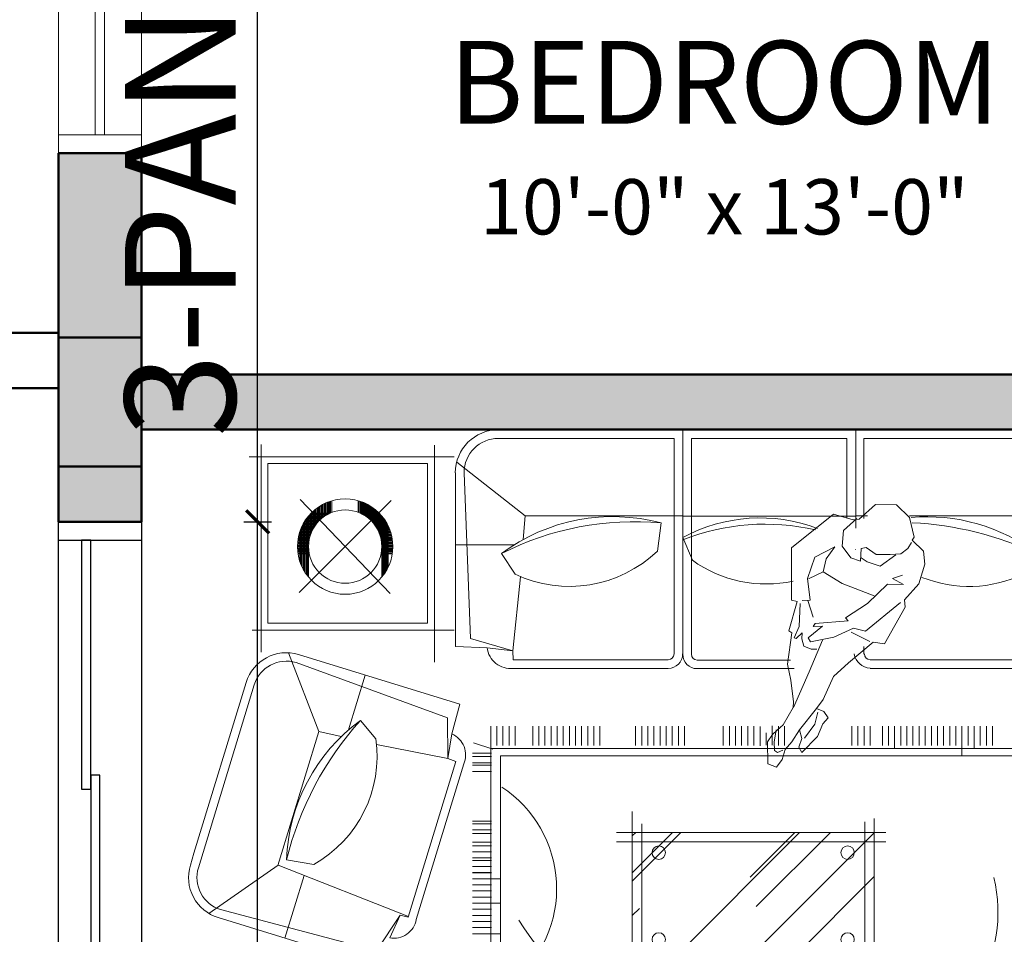
# Model space of a CAD drawing. Units: inches. Extents: x 375 to 1122, y 27 to 1069.
# Tile 69 of 155: x 494 to 601, y 400 to 499. Entities that reach past the tile are written whole.
import ezdxf

# ---------------------------------------------------------------- set-up
doc = ezdxf.new("R2010")
doc.units = ezdxf.units.IN
for name, color, linetype, lineweight in [('A-ANNO-DIMS', 2, 'Continuous', 18), ('A-AREA-IDEN', 7, 'Continuous', 18), ('A-COLS-PATT', 10, 'Continuous', 13), ('A-WALL-PATT', 252, 'Continuous', 13), ('Columns', 10, 'Continuous', 50), ('Doors', 150, 'Continuous', 25), ('Furniture', 30, 'Continuous', 18), ('Walls', 250, 'Continuous', 50), ('Windows', 122, 'Continuous', 18)]:
    doc.layers.add(name, color=color, linetype=linetype, lineweight=lineweight)
doc.styles.get("Standard").update_dxf_attribs({"font": 'arial.ttf'})
doc.dimstyles.new('ISO-25', dxfattribs={"dimtxt": 12, "dimasz": 2.5, "dimexe": 1.5, "dimexo": 1.5, "dimtad": 1, "dimdec": 1, "dimlunit": 3, "dimtxsty": 'Standard', "dimblk": 'ARCHTICK', "dimcen": 2.5, "dimadec": 0, "dimazin": 0, "dimtfac": 1, "dimtdec": 1, "dimtmove": 0, "dimatfit": 3, "dimfxl": 1.5, "dimfxlon": 1, "dimarcsym": 0})

# ---------------------------------------------------------------- blocks, each defined once
blk = doc.blocks.new('A$C4DC51D13')
for p, q in [((3265.3, 2996.2), (1188.4, 2996.2)), ((1895.2, 2134), (1895.2, 2996.2)), ((2559.6, 2996.2), (2559.6, 2617.8)), ((1188.4, 2962.7), (1862.1, 2962.7)), ((1862.1, 2134), (1862.1, 2962.7)), ((1928.3, 2961.6), (2524.2, 2961.6)), ((1928.3, 2134), (1928.3, 2961.6)), ((2524.2, 2961.6), (2524.2, 2658.6)), ((2590.4, 2962.7), (2590.4, 2654.5)), ((3265.3, 2962.7), (2590.4, 2962.7)), ((277.4, 2939.6), (277.4, 2141.8)), ((943, 2103.5), (943, 2936.7)), ((1018.2, 2892.3), (232.2, 2892.3)), ((1290.4, 2664.8), (1028, 2870.9)), ((304, 2865.7), (304, 2253.3)), ((916.4, 2865.7), (304, 2865.7)), ((916.4, 2253.3), (916.4, 2865.7)), ((1022.9, 2163.8), (1022.9, 2830.3)), ((1056, 2830.3), (1081, 2194.8)), ((423.7, 2370.8), (776.6, 2723.7)), ((427.4, 2727.4), (772.8, 2367.1)), ((540.2, 2674.6), (540.2, 2720.2)), ((544.4, 2676.5), (544.4, 2721.6)), ((548.7, 2678.2), (548.7, 2722.9)), ((650.1, 2678.8), (650.1, 2723.3)), ((654.3, 2677.1), (654.3, 2722)), ((658.6, 2675.2), (658.6, 2720.7)), ((476.8, 2615), (476.8, 2682.5)), ((481, 2622.2), (481, 2686.2)), ((485.3, 2628.5), (485.3, 2689.7)), ((489.5, 2634.2), (489.5, 2693)), ((493.7, 2639.3), (493.7, 2696.1)), ((497.9, 2644), (497.9, 2699.1)), ((502.2, 2648.3), (502.2, 2701.8)), ((506.4, 2652.2), (506.4, 2704.4)), ((510.6, 2655.8), (510.6, 2706.9)), ((514.9, 2659.2), (514.9, 2709.2)), ((519.1, 2662.3), (519.1, 2711.3)), ((523.3, 2665.1), (523.3, 2713.4)), ((527.5, 2667.8), (527.5, 2715.2)), ((531.8, 2670.2), (531.8, 2717)), ((536, 2672.5), (536, 2718.7)), ((662.8, 2673.2), (662.8, 2719.2)), ((667, 2671), (667, 2717.6)), ((668.5, 2670.2), (668.5, 2717)), ((671.2, 2668.6), (671.2, 2715.9)), ((672.7, 2667.8), (672.7, 2715.2)), ((675.5, 2666.1), (675.5, 2714)), ((676.9, 2665.1), (676.9, 2713.4)), ((679.7, 2663.3), (679.7, 2712)), ((681.1, 2662.3), (681.1, 2711.3)), ((683.9, 2660.3), (683.9, 2709.9)), ((685.4, 2659.2), (685.4, 2709.2)), ((688.1, 2657), (688.1, 2707.7)), ((689.6, 2655.8), (689.6, 2706.9)), ((692.4, 2653.5), (692.4, 2705.3)), ((693.8, 2652.2), (693.8, 2704.4)), ((696.6, 2649.6), (696.6, 2702.7)), ((698, 2648.3), (698, 2701.8)), ((700.8, 2645.5), (700.8, 2700)), ((702.3, 2644), (702.3, 2699.1)), ((705, 2641), (705, 2697.2)), ((706.5, 2639.3), (706.5, 2696.1)), ((709.3, 2636), (709.3, 2694.1)), ((710.7, 2634.2), (710.7, 2693)), ((713.5, 2630.5), (713.5, 2690.9)), ((714.9, 2628.5), (714.9, 2689.7)), ((717.7, 2624.4), (717.7, 2687.4)), ((719.2, 2622.2), (719.2, 2686.2)), ((722, 2617.6), (722, 2683.8)), ((723.4, 2615), (723.4, 2682.5)), ((446.1, 2646.1), (500, 2646.1)), ((447.2, 2446.7), (447.2, 2647.8)), ((448.9, 2650.4), (504.4, 2650.4)), ((451.5, 2440.6), (451.5, 2654)), ((451.9, 2654.6), (509.2, 2654.6)), ((455.1, 2658.8), (514.4, 2658.8)), ((455.7, 2434.9), (455.7, 2659.6)), ((458.4, 2663.1), (520.2, 2663.1)), ((459.9, 2558.8), (459.9, 2664.9)), ((462, 2667.3), (526.7, 2667.3)), ((464.1, 2583.3), (464.1, 2669.7)), ((465.8, 2671.5), (534.1, 2671.5)), ((468.4, 2596.6), (468.4, 2674.3)), ((469.8, 2675.7), (542.8, 2675.7)), ((472.6, 2606.7), (472.6, 2678.5)), ((489.5, 2667.3), (489.5, 2633.5)), ((657.4, 2675.7), (730.4, 2675.7)), ((734.5, 2671.5), (666.1, 2671.5)), ((666.1, 2671.5), (734.5, 2671.5)), ((738.2, 2667.3), (673.5, 2667.3)), ((673.5, 2667.3), (738.2, 2667.3)), ((741.8, 2663.1), (680, 2663.1)), ((680, 2663.1), (741.8, 2663.1)), ((745.2, 2658.8), (685.8, 2658.8)), ((685.8, 2658.8), (745.2, 2658.8)), ((748.3, 2654.6), (691, 2654.6)), ((691, 2654.6), (748.3, 2654.6)), ((751.3, 2650.4), (695.8, 2650.4)), ((695.8, 2650.4), (751.3, 2650.4)), ((754.1, 2646.1), (700.2, 2646.1)), ((700.2, 2646.1), (754.1, 2646.1)), ((726.2, 2609.7), (726.2, 2679.9)), ((727.6, 2606.7), (727.6, 2678.5)), ((730.4, 2600.3), (730.4, 2675.7)), ((731.9, 2596.6), (731.9, 2674.3)), ((734.6, 2588.4), (734.6, 2671.3)), ((736.1, 2583.3), (736.1, 2669.7)), ((738.9, 2570.4), (738.9, 2666.6)), ((740.3, 2558.8), (740.3, 2664.9)), ((743.1, 2433.1), (743.1, 2661.5)), ((744.5, 2434.9), (744.5, 2659.6)), ((747.3, 2438.6), (747.3, 2656)), ((748.8, 2440.6), (748.8, 2654)), ((751.5, 2444.5), (751.5, 2650)), ((753, 2446.7), (753, 2647.8)), ((1283.3, 2574.2), (1290.4, 2664.8)), ((1290.4, 2664.8), (1894.7, 2664.8)), ((1895.2, 2663.7), (2557.3, 2663.7)), ((2603.6, 2664.8), (2559, 2664.8)), ((3163.3, 2664.8), (2764.7, 2664.8)), ((427.5, 2608.1), (473.3, 2608.1)), ((429.1, 2612.3), (475.4, 2612.3)), ((430.3, 2479), (430.3, 2615.5)), ((430.7, 2616.6), (477.7, 2616.6)), ((432.5, 2620.8), (480.2, 2620.8)), ((434.5, 2469.3), (434.5, 2625.2)), ((434.5, 2625), (482.9, 2625)), ((436.5, 2629.2), (485.8, 2629.2)), ((438.7, 2633.5), (488.9, 2633.5)), ((438.8, 2460.9), (438.8, 2633.6)), ((441, 2637.7), (492.3, 2637.7)), ((443, 2453.4), (443, 2641.1)), ((443.5, 2641.9), (496, 2641.9)), ((756.7, 2641.9), (704.2, 2641.9)), ((704.2, 2641.9), (756.7, 2641.9)), ((759.2, 2637.7), (707.9, 2637.7)), ((707.9, 2637.7), (759.2, 2637.7)), ((761.5, 2633.5), (711.3, 2633.5)), ((711.3, 2633.5), (761.5, 2633.5)), ((763.7, 2629.2), (714.4, 2629.2)), ((714.4, 2629.2), (763.7, 2629.2)), ((765.8, 2625), (717.3, 2625)), ((767.7, 2620.8), (720, 2620.8)), ((769.5, 2616.6), (722.5, 2616.6)), ((771.1, 2612.3), (724.8, 2612.3)), ((772.7, 2608.1), (726.9, 2608.1)), ((755.8, 2451.1), (755.8, 2643.5)), ((757.2, 2453.4), (757.2, 2641.1)), ((760, 2458.3), (760, 2636.3)), ((761.4, 2460.9), (761.4, 2633.6)), ((764.2, 2466.3), (764.2, 2628.2)), ((765.7, 2469.3), (765.7, 2625.2)), ((1798, 2530.2), (1812.1, 2637.9)), ((418.5, 2570.1), (461.3, 2570.1)), ((419.1, 2574.3), (462.1, 2574.3)), ((419.8, 2578.5), (462.9, 2578.5)), ((420.6, 2582.7), (464, 2582.7)), ((421.5, 2587), (465.2, 2587)), ((422.5, 2591.2), (466.5, 2591.2)), ((423.6, 2595.4), (467.9, 2595.4)), ((424.8, 2599.7), (469.6, 2599.7)), ((426.1, 2603.9), (471.3, 2603.9)), ((426.1, 2490.7), (426.1, 2603.9)), ((774.1, 2603.9), (728.9, 2603.9)), ((775.4, 2599.7), (730.7, 2599.7)), ((776.6, 2595.4), (732.3, 2595.4)), ((777.7, 2591.2), (733.7, 2591.2)), ((778.7, 2587), (735.1, 2587)), ((779.6, 2582.7), (736.2, 2582.7)), ((780.4, 2578.5), (737.3, 2578.5)), ((781.1, 2574.3), (738.2, 2574.3)), ((781.7, 2570.1), (738.9, 2570.1)), ((1895.5, 2582.2), (1932.3, 2494.6)), ((417.1, 2548.9), (459.4, 2548.9)), ((417.1, 2544.7), (459.5, 2544.7)), ((417.2, 2553.2), (459.6, 2553.2)), ((417.2, 2540.5), (459.6, 2540.5)), ((417.4, 2557.4), (459.8, 2557.4)), ((417.5, 2536.3), (459.9, 2536.3)), ((417.7, 2561.6), (460.2, 2561.6)), ((417.8, 2532), (460.3, 2532)), ((418.1, 2565.8), (460.7, 2565.8)), ((459.9, 2429.7), (459.9, 2535.7)), ((782.2, 2565.8), (739.6, 2565.8)), ((782.5, 2532), (740, 2532)), ((782.5, 2561.6), (740.1, 2561.6)), ((740.3, 2429.7), (740.3, 2535.7)), ((782.8, 2557.4), (740.4, 2557.4)), ((782.8, 2536.3), (740.4, 2536.3)), ((783, 2540.5), (740.6, 2540.5)), ((783, 2553.2), (740.7, 2553.2)), ((783.1, 2548.9), (740.8, 2548.9)), ((783.1, 2544.7), (740.8, 2544.7)), ((1022.9, 2554.4), (1249.6, 2554.4)), ((2559, 2535.8), (2557.3, 2535.8)), ((418.2, 2527.8), (460.8, 2527.8)), ((418.7, 2523.6), (461.4, 2523.6)), ((419.3, 2519.4), (462.2, 2519.4)), ((781, 2519.4), (738, 2519.4)), ((781.6, 2523.6), (738.8, 2523.6)), ((782.1, 2527.8), (739.4, 2527.8)), ((1200, 2520.5), (1251.9, 2440.8)), ((1243.2, 2146.7), (1272.2, 2431.8)), ((304, 2253.3), (916.4, 2253.3)), ((242.9, 2226.7), (1018.2, 2226.7)), ((1081, 2194.8), (1243.2, 2146.7)), ((1145.1, 2159.3), (1022.9, 2163.8)), ((1145.1, 2159.3), (1243.2, 2146.7)), ((2590.4, 2164.3), (2590.4, 2134)), ((498.8, 1837.1), (382.1, 2139.5)), ((1040.3, 1942.9), (421.2, 2132.6)), ((1244.8, 2113), (1243.2, 2146.7)), ((411.8, 2101.9), (992.6, 1890.2)), ((1839.5, 2113), (1244.8, 2113)), ((1839.5, 2079.9), (1244.8, 2079.9)), ((2308.5, 2111.9), (1950.4, 2111.9)), ((2322.1, 2078.8), (1950.4, 2078.8)), ((2614.2, 2113), (3208.9, 2113)), ((2614.2, 2079.9), (3208.9, 2079.9)), ((677.4, 2054.1), (612.9, 1843.6)), ((220.3, 2026), (19.3, 1370.1)), ((251.1, 2016.6), (37.1, 1314.7)), ((1009.7, 1828.1), (1040.3, 1942.9)), ((992.6, 1890.2), (993.4, 1733.4)), ((658.5, 1880), (717.8, 1809.1)), ((1158.3, 1784.3), (1158.3, 1858.2)), ((1181.8, 1784.3), (1181.8, 1858.2)), ((1205.3, 1784.3), (1205.3, 1858.2)), ((1228.8, 1784.3), (1228.8, 1858.2)), ((1252.2, 1784.3), (1252.2, 1858.2)), ((1319.4, 1784.3), (1319.4, 1858.2)), ((1342.9, 1784.3), (1342.9, 1858.2)), ((1366.3, 1784.3), (1366.3, 1858.2)), ((1389.8, 1784.3), (1389.8, 1858.2)), ((1413.3, 1784.3), (1413.3, 1858.2)), ((1436.8, 1784.3), (1436.8, 1858.2)), ((1460.2, 1784.3), (1460.2, 1858.2)), ((1483.7, 1784.3), (1483.7, 1858.2)), ((1507.2, 1784.3), (1507.2, 1858.2)), ((1530.7, 1784.3), (1530.7, 1858.2)), ((1554.1, 1784.3), (1554.1, 1858.2)), ((1577.6, 1784.3), (1577.6, 1858.2)), ((1714.2, 1784.3), (1714.2, 1858.2)), ((1737.6, 1784.3), (1737.6, 1858.2)), ((1761.1, 1784.3), (1761.1, 1858.2)), ((1784.6, 1784.3), (1784.6, 1858.2)), ((1808.1, 1784.3), (1808.1, 1858.2)), ((1831.5, 1784.3), (1831.5, 1858.2)), ((1855, 1784.3), (1855, 1858.2)), ((1878.5, 1784.3), (1878.5, 1858.2)), ((1902, 1784.3), (1902, 1858.2)), ((2050.7, 1784.3), (2050.7, 1858.2)), ((2074.2, 1784.3), (2074.2, 1858.2)), ((2097.7, 1784.3), (2097.7, 1858.2)), ((2121.1, 1784.3), (2121.1, 1858.2)), ((2144.6, 1784.3), (2144.6, 1858.2)), ((2168.1, 1784.3), (2168.1, 1858.2)), ((2191.6, 1782.4), (2191.6, 1856.3)), ((2238.5, 1785.1), (2238.5, 1859)), ((2262, 1784.3), (2262, 1858.2)), ((2285.4, 1784.3), (2285.4, 1858.2)), ((2543.7, 1784.3), (2543.7, 1858.2)), ((2567.1, 1784.3), (2567.1, 1858.2)), ((2590.6, 1784.3), (2590.6, 1858.2)), ((2614.1, 1784.3), (2614.1, 1858.2)), ((2661, 1784.3), (2661, 1858.2)), ((2684.5, 1784.3), (2684.5, 1858.2)), ((2708, 1772.3), (2708, 1858.2)), ((2731.5, 1784.3), (2731.5, 1858.2)), ((2754.9, 1784.3), (2754.9, 1858.2)), ((2778.4, 1784.3), (2778.4, 1858.2)), ((2801.9, 1784.3), (2801.9, 1858.2)), ((2825.4, 1784.3), (2825.4, 1858.2)), ((2848.8, 1784.3), (2848.8, 1858.2)), ((2872.3, 1784.3), (2872.3, 1858.2)), ((2895.8, 1784.3), (2895.8, 1858.2)), ((2919.3, 1784.3), (2919.3, 1858.2)), ((2942.7, 1784.3), (2942.7, 1858.2)), ((2966.2, 1744.8), (2966.2, 1858.2)), ((2989.7, 1784.3), (2989.7, 1858.2)), ((3013.2, 1772.3), (3013.2, 1858.2)), ((3036.6, 1784.3), (3036.6, 1858.2)), ((3060.1, 1784.3), (3060.1, 1858.2)), ((3083.6, 1784.3), (3083.6, 1858.2)), ((498.8, 1837.1), (341.4, 1323.6)), ((584.9, 1817.9), (498.8, 1837.1)), ((1009.7, 1828.1), (993.4, 1733.4)), ((1158.3, 1821.3), (1158.5, 487.7)), ((2215, 1785.7), (2215, 1832.3)), ((993.4, 1733.4), (720.4, 1787.6)), ((1166.1, 1769.7), (1091.8, 1794.5)), ((1162.1, 1754.9), (1088.2, 1754.9)), ((1162.1, 1741.1), (1088.2, 1741.1)), ((3248.4, 1772.3), (1158.5, 1772.3)), ((1196, 511), (1196, 1744.8)), ((1196, 1744.8), (3215.6, 1744.8)), ((1024.2, 1722.3), (842.3, 1125.2)), ((873.1, 1115.8), (1055, 1712.9)), ((1024.2, 1722.3), (993.4, 1733.4)), ((1162.1, 1717.6), (1088.2, 1717.6)), ((1162.1, 1708), (1088.2, 1708)), ((1162.1, 1684.5), (1088.2, 1684.5)), ((1701.7, 1530), (1701.7, 911.2)), ((1162.1, 1492.9), (1088.2, 1492.9)), ((1162.1, 1483.3), (1088.2, 1483.3)), ((1737.7, 1483.1), (1737.7, 911.2)), ((2593.1, 907.9), (2593.1, 1490.3)), ((2629.1, 907.9), (2629.1, 1503.1)), ((1162.1, 1459.8), (1088.2, 1459.8)), ((1162.1, 1446), (1088.2, 1446)), ((2674.6, 1449.9), (1641, 1449.9)), ((1888.1, 1449.9), (1701.7, 1263.5)), ((1856.2, 1449.9), (1701.7, 1295.4)), ((1715.1, 1449.9), (1701.7, 1436.5)), ((2343.3, 1449.9), (1855.3, 961.9)), ((2629.1, 1449), (2142, 961.9)), ((2325.1, 1449.9), (2154.2, 1279.1)), ((2461.6, 1449.9), (2177, 1165.3)), ((1162.1, 1412.8), (1088.2, 1412.8)), ((1162.1, 1399), (1088.2, 1399)), ((2674.6, 1413.9), (1641, 1413.9)), ((6.3, 1324.2), (19.3, 1370.2)), ((1162.1, 1375.5), (1088.2, 1375.5)), ((342.8, 1324.6), (76.7, 1139.6)), ((843, 1127.6), (342.8, 1324.6)), ((479.3, 1327.3), (375.2, 1344.9)), ((1162.1, 1352.1), (1088.2, 1352.1)), ((1162.1, 1342.9), (1088.2, 1342.9)), ((1162.1, 1342.4), (1088.2, 1342.4)), ((369.2, 1044.8), (442.9, 1285.2)), ((1162.1, 1319.4), (1088.2, 1319.4)), ((1162.1, 1318.9), (1088.2, 1318.9)), ((1162.1, 1296), (1088.2, 1296)), ((1162.1, 1295.5), (1088.2, 1295.5)), ((1196, 1272.5), (1088.2, 1272.5)), ((1162.1, 1272), (1088.2, 1272)), ((1162.1, 1249), (1088.2, 1249)), ((1162.1, 1248.5), (1088.2, 1248.5)), ((2629.1, 1280.5), (2310.5, 961.9)), ((1162.1, 1225.5), (1088.2, 1225.5)), ((1162.1, 1202.1), (1088.2, 1202.1)), ((1196, 1178.6), (1088.2, 1178.6)), ((122.4, 1154.1), (719.7, 996.3)), ((719.7, 996.3), (810.6, 1133.2)), ((771, 1045.7), (810.6, 1133.2)), ((842.3, 1125.2), (810.6, 1133.2)), ((1162.1, 1155.1), (1088.2, 1155.1)), ((1728.6, 1158.4), (1701.7, 1131.5)), ((732, 933.5), (112.9, 1123.3)), ((1162.1, 1131.6), (1088.2, 1131.6)), ((1162.1, 1108.2), (1088.2, 1108.2)), ((1162.1, 1084.7), (1088.2, 1084.7)), ((1196, 1061.2), (1088.2, 1061.2))]:
    blk.add_line(p, q)
at = {"linetype": 'ByBlock'}
blk.add_lwpolyline([(2342.9, 1843.9), (2352.5, 1810.4), (2340.1, 1777.7), (2351.8, 1757), (2412.3, 1818), (2433.1, 1866.4), (2453.1, 1889.5), (2436, 1914.7), (2407.6, 1926.2), (2433.7, 1959.9), (2473.1, 2048.3), (2530.6, 2101.1), (2625.9, 2180.3), (2669, 2174.2), (2748.1, 2315.4), (2745.8, 2342.6), (2801.2, 2404.9), (2823.9, 2479.6), (2818.4, 2529.9), (2775.1, 2571.7), (2782.4, 2583.3), (2765.2, 2658.8), (2714.5, 2706.9), (2634.6, 2708.6), (2571.9, 2652.6), (2548.8, 2649.4), (2474, 2672.1), (2312.9, 2542.1), (2312.9, 2341.6), (2333.9, 2336.4), (2302, 2223.9), (2313.6, 2216.6), (2297.4, 2095.7), (2309.3, 2034.9), (2320.2, 1952), (2319.3, 1929.9), (2280.8, 1863.6), (2257.7, 1842.4), (2239.2, 1825.7), (2220.1, 1798.2), (2221.6, 1713.1), (2254.3, 1700.7), (2275.9, 1729.8), (2288.6, 1768), (2313.7, 1797.6)], close=True, dxfattribs=at)
for points in [[(2563.4, 2654.7), (2512.2, 2609.3), (2506.2, 2548.3), (2540.1, 2504.4), (2576.9, 2490.9), (2579.8, 2539.3), (2598.7, 2543.6), (2636.7, 2516.4), (2690.3, 2516.7), (2731.2, 2520.1), (2758.5, 2540.1), (2773, 2563.3)], [(2629.1, 2357.8), (2507, 2405.5), (2433.2, 2450.3), (2445.5, 2500.8), (2478.9, 2546.1), (2402.4, 2506.9), (2373.4, 2424.8), (2384.4, 2341.9), (2352.8, 2340.7)], [(2712.3, 2515.8), (2652.7, 2472.4), (2603.2, 2489), (2580, 2503.6)], [(2738, 2438.2), (2699.2, 2425.4), (2742.4, 2401.4), (2680.4, 2403.2), (2604.1, 2328.3), (2519.2, 2273.3), (2529.8, 2261.8), (2402.7, 2252.7), (2395.4, 2241.1), (2431.1, 2241.3), (2375.7, 2196.9), (2385.2, 2181.2), (2474.4, 2199.5), (2549.9, 2234.6), (2596.2, 2223.2), (2730.1, 2333.1)], [(2433.2, 2450.3), (2377.6, 2423.8)], [(2409.5, 2153), (2387.5, 2153.9), (2359, 2165.4), (2352.6, 2193.7), (2353.5, 2215.7), (2330.5, 2194.6), (2322.1, 2196.7), (2341.8, 2240.9), (2345.5, 2329.1)], [(2374.9, 2339.8), (2395.2, 2276.9)], [(2613.2, 2183.4), (2541.6, 2218.8)], [(2431.4, 2187.8), (2379.5, 2066.7), (2320.2, 1929.7)], [(2407.6, 1926.2), (2342.9, 1843.9)], [(2412.9, 1911.5), (2401.6, 1865.2), (2361.9, 1812.5)], [(2279.2, 1765.9), (2259.2, 1757.4), (2247.6, 1764.7), (2246.4, 1796.2), (2253.5, 1843.5)]]:
    blk.add_lwpolyline(points, dxfattribs=at)
for centre, radius in [((600.1, 2547.3), 183), ((600.1, 2547.3), 140.7), ((1803.2, 1372.6), 25.7), ((2527.6, 1372.6), 25.7), ((1803.2, 1039.3), 25.7), ((2527.6, 1039.3), 25.7)]:
    blk.add_circle(centre, radius)
for centre, radius, start, end in [((1188.4, 2830.3), 165.9, 90, 180), ((1188.4, 2830.3), 132.4, 90, 180), ((1626.8, 1949.8), 712.7, 74.928, 126.7929), ((2192.2, 2032.6), 624.6, 69.4145, 118.3621), ((2633.9, 373.6), 2292.5, 91.8726, 91.9144), ((2832.8, 1963.1), 698.5, 52.9389, 95.0789), ((1707.9, 1527), 1115.8, 84.6406, 117.0804), ((2210.2, 1780.8), 852.5, 76.866, 111.6839), ((2713.3, 1357.7), 1282.3, 65.0725, 87.2152), ((1459.9, 2882.7), 488.4, 244.7866, 313.8058), ((2216, 2892.1), 488.4, 234.4888, 282.1285), ((2993.8, 2882.7), 488.4, 248.2152, 295.2134), ((1234.5, 2169.3), 90, 186.4251, 276.5821), ((374.1, 1978.9), 160.8, 72.9571, 162.9571), ((1839.5, 2135.1), 22.1, 270, 0), ((1839.5, 2135.1), 55.2, 270, 0), ((1950.4, 2134), 55.2, 180, 270), ((1950.4, 2134), 22.1, 180, 270), ((2619.6, 2148.3), 68.5, 191.0595, 265.4426), ((2614.2, 2135.1), 22.1, 180, 270), ((374.1, 1978.9), 128.6, 72.9571, 162.9571), ((1584.7, 1047), 1245.7, 138.0296, 166.1636), ((1067.1, 1321), 692.3, 126.1642, 178.0291), ((974.8, 1747.9), 87.4, 336.375, 66.532), ((248.2, 1741.7), 474.4, 299.1514, 8.1705), ((944.2, 1233.8), 467.1, 309.4804, 56.621), ((160.1, 1277), 160.8, 162.9571, 252.9571), ((160.1, 1277), 128.6, 162.9571, 252.9571), ((2517.5, 1143.6), 586.7, 287.3395, 13.1463), ((787.1, 1131.7), 87.4, 259.3822, 349.5393), ((2356.9, 1798.1), 1287.8, 212.1153, 261.9323)]:
    blk.add_arc(centre, radius, start, end)
blk = doc.blocks.new('WINDOW-72IN')
for p, q in [((4, 70), (4, 2)), ((5, 70), (5, 2))]:
    blk.add_line(p, q)
blk.add_lwpolyline([(9, 0), (0, 0), (0, 72), (9, 72)], close=True)
for points in [[(0, 70), (9, 70)], [(9, 2), (0, 2)]]:
    blk.add_lwpolyline(points)
blk = doc.blocks.new('BALCONY-SLIDER-3P-84IN')
for points in [[(0, 84), (9, 84), (9, 0), (0, 0)], [(2.5, 55), (3.5, 55), (3.5, 82), (2.5, 82)], [(3.5, 28), (4.5, 28), (4.5, 56.5), (3.5, 56.5)], [(4.5, 2), (5.5, 2), (5.5, 29), (4.5, 29)]]:
    blk.add_lwpolyline(points, close=True)
for points in [[(0, 82), (9, 82)], [(9, 2), (0, 2)]]:
    blk.add_lwpolyline(points)
blk = doc.blocks.new('COLUMN-14X9IN')
blk.add_lwpolyline([(0, 0), (14, 0), (14, 9), (0, 9)], close=True)
blk = doc.blocks.new('_ArchTick')
at = {"color": 0, "linetype": 'ByBlock', "const_width": 0.15}
blk.add_lwpolyline([(-0.5, -0.5), (0.5, 0.5)], dxfattribs=at)
blk = doc.blocks.new('*D44')
at = {"layer": 'A-ANNO-DIMS', "color": 0, "lineweight": -2, "transparency": 16777216}
for p, q in [((541.85, 504.43), (541.85, 501.43)), ((607.16, 504.43), (607.16, 501.43)), ((541.85, 502.93), (607.16, 502.93)), ((607.16, 502.93), (712.02, 502.93))]:
    blk.add_line(p, q, dxfattribs=at)
at = {"layer": 'Defpoints', "color": 0, "transparency": 16777216}
for p in [(541.85, 513.06), (607.16, 513.06), (607.16, 502.93)]:
    blk.add_point(p, dxfattribs=at)
at = {"layer": 'A-ANNO-DIMS', "color": 0, "lineweight": -2, "transparency": 16777216, "xscale": 2.5, "yscale": 2.5, "zscale": 2.5, "rotation": 180}
blk.add_blockref('_ArchTick', (541.85, 502.93), dxfattribs=at)
at = {"layer": 'A-ANNO-DIMS', "color": 0, "lineweight": -2, "transparency": 16777216, "xscale": 2.5, "yscale": 2.5, "zscale": 2.5}
blk.add_blockref('_ArchTick', (607.16, 502.93), dxfattribs=at)
at = {"layer": 'A-ANNO-DIMS', "color": 0, "transparency": 16777216, "insert": (660.84, 509.76), "char_height": 12, "attachment_point": 5}
blk.add_mtext('5\'-5 1/2" TYP.', dxfattribs=at)
blk = doc.blocks.new('*D71')
at = {"layer": 'A-ANNO-DIMS', "color": 0, "lineweight": -2, "transparency": 16777216}
for p, q in [((520.11, 444.53), (520.11, 661.17)), ((518.61, 444.53), (521.61, 444.53)), ((520.11, 360.53), (520.11, 444.53)), ((518.61, 360.53), (521.61, 360.53))]:
    blk.add_line(p, q, dxfattribs=at)
at = {"layer": 'Defpoints', "color": 0, "transparency": 16777216}
for p in [(507.51, 444.53), (520.11, 444.53), (507.51, 360.53)]:
    blk.add_point(p, dxfattribs=at)
at = {"layer": 'A-ANNO-DIMS', "color": 0, "lineweight": -2, "transparency": 16777216, "xscale": 2.5, "yscale": 2.5, "zscale": 2.5}
for p, rotation in [((520.11, 444.53), 90), ((520.11, 360.53), 270)]:
    blk.add_blockref('_ArchTick', p, dxfattribs=dict(at, rotation=rotation))
at = {"layer": 'A-ANNO-DIMS', "color": 0, "transparency": 16777216, "insert": (513.27, 554.1), "char_height": 12, "attachment_point": 5, "rotation": 90}
blk.add_mtext('3-PANEL SLIDER 7\'-0" TYP.', dxfattribs=at)
blk = doc.blocks.new('*D82')
at = {"layer": 'A-ANNO-DIMS', "color": 0, "lineweight": -2, "transparency": 16777216}
for p, q in [((401.51, 1009.53), (398.51, 1009.53)), ((400.01, 160.53), (400.01, 1009.53)), ((401.51, 160.53), (398.51, 160.53))]:
    blk.add_line(p, q, dxfattribs=at)
at = {"layer": 'Defpoints', "color": 0, "transparency": 16777216}
for p in [(400.01, 1009.53), (630.53, 1009.53), (630.53, 160.53)]:
    blk.add_point(p, dxfattribs=at)
at = {"layer": 'A-ANNO-DIMS', "color": 0, "lineweight": -2, "transparency": 16777216, "xscale": 2.5, "yscale": 2.5, "zscale": 2.5}
for p, rotation in [((400.01, 1009.53), 90), ((400.01, 160.53), 270)]:
    blk.add_blockref('_ArchTick', p, dxfattribs=dict(at, rotation=rotation))
at = {"layer": 'A-ANNO-DIMS', "color": 0, "transparency": 16777216, "insert": (393.26, 585.03), "char_height": 12, "attachment_point": 5, "rotation": 90}
blk.add_mtext('70\'-9"', dxfattribs=at)

msp = doc.modelspace()

# ---------------------------------------------------------------- hatches: boundary and pattern name
at = {"layer": 'A-COLS-PATT'}
h = msp.add_hatch(color=256, dxfattribs=at)
h.dxf.hatch_style = 1
h.paths.add_polyline_path([(512.51, 982.53), (498.51, 982.53), (498.51, 973.53), (512.51, 973.53)])
h.paths.add_polyline_path([(666.51, 982.53), (652.51, 982.53), (652.51, 973.53), (666.51, 973.53)])
h.paths.add_polyline_path([(802.01, 982.53), (788.01, 982.53), (788.01, 973.53), (802.01, 973.53)])
h.paths.add_polyline_path([(932.01, 982.53), (918.01, 982.53), (918.01, 973.53), (932.01, 973.53)])
h.paths.add_polyline_path([(507.51, 841.53), (498.51, 841.53), (498.51, 827.53), (507.51, 827.53)])
h.paths.add_polyline_path([(666.51, 844.53), (652.51, 844.53), (652.51, 835.53), (666.51, 835.53)])
h.paths.add_polyline_path([(802.01, 814.53), (788.01, 814.53), (788.01, 805.53), (802.01, 805.53)])
h.paths.add_polyline_path([(932.01, 814.53), (918.01, 814.53), (918.01, 805.53), (932.01, 805.53)])
h.paths.add_polyline_path([(507.51, 719.53), (498.51, 719.53), (498.51, 705.53), (507.51, 705.53)])
h.paths.add_polyline_path([(731.01, 676.53), (722.01, 676.53), (722.01, 662.53), (731.01, 662.53)])
h.paths.add_polyline_path([(802.01, 676.53), (788.01, 676.53), (788.01, 667.53), (802.01, 667.53)])
h.paths.add_polyline_path([(932.01, 676.53), (918.01, 676.53), (918.01, 667.53), (932.01, 667.53)])
h.paths.add_polyline_path([(932.01, 583.53), (918.01, 583.53), (918.01, 574.53), (932.01, 574.53)])
h.paths.add_polyline_path([(868.01, 583.53), (854.01, 583.53), (854.01, 574.53), (868.01, 574.53)])
h.paths.add_polyline_path([(868.01, 502.53), (854.01, 502.53), (854.01, 493.53), (868.01, 493.53)])
h.paths.add_polyline_path([(932.01, 502.53), (918.01, 502.53), (918.01, 493.53), (932.01, 493.53)])
h.paths.add_polyline_path([(672.51, 592.03), (663.51, 592.03), (663.51, 578.03), (672.51, 578.03)])
h.paths.add_polyline_path([(512.51, 589.53), (498.51, 589.53), (498.51, 580.53), (512.51, 580.53)])
h.paths.add_polyline_path([(507.51, 464.53), (498.51, 464.53), (498.51, 450.53), (507.51, 450.53)])
h.paths.add_polyline_path([(731.01, 507.53), (722.01, 507.53), (722.01, 493.53), (731.01, 493.53)])
h.paths.add_polyline_path([(802.01, 502.53), (788.01, 502.53), (788.01, 493.53), (802.01, 493.53)])
h.paths.add_polyline_path([(507.51, 342.53), (498.51, 342.53), (498.51, 328.53), (507.51, 328.53)])
h.paths.add_polyline_path([(512.51, 196.53), (498.51, 196.53), (498.51, 187.53), (512.51, 187.53)])
h.paths.add_polyline_path([(666.51, 334.53), (652.51, 334.53), (652.51, 325.53), (666.51, 325.53)])
h.paths.add_polyline_path([(666.51, 196.53), (652.51, 196.53), (652.51, 187.53), (666.51, 187.53)])
h.paths.add_polyline_path([(805.01, 196.53), (791.01, 196.53), (791.01, 187.53), (805.01, 187.53)])
h.paths.add_polyline_path([(932.01, 196.53), (918.01, 196.53), (918.01, 187.53), (932.01, 187.53)])
h.paths.add_polyline_path([(932.01, 334.53), (918.01, 334.53), (918.01, 325.53), (932.01, 325.53)])
h.paths.add_polyline_path([(805.01, 334.53), (791.01, 334.53), (791.01, 325.53), (805.01, 325.53)])
at = {"layer": 'A-WALL-PATT'}
h = msp.add_hatch(color=256, dxfattribs=at)
h.dxf.hatch_style = 1
h.paths.add_polyline_path([(962.01, 388.53), (989.01, 388.53), (989.01, 394.53), (962.01, 394.53), (932.01, 394.53), (932.01, 397.53), (923.01, 397.53), (923.01, 394.53), (842.01, 394.53), (842.01, 334.53), (839.51, 334.53), (839.51, 328.53), (854.01, 328.53), (854.01, 334.53), (848.01, 334.53), (848.01, 388.53), (953.01, 388.53), (953.01, 356.08), (962.01, 356.08), (962.01, 358.55), (989.01, 358.55), (989.01, 364.55), (962.01, 364.55)])
h.paths.add_polyline_path([(989.01, 502.53), (932.01, 502.53), (932.01, 583.53), (932.01, 593.53), (923.01, 593.53), (923.01, 583.53), (854.01, 583.53), (854.01, 556.53), (863.01, 556.53), (863.01, 574.53), (923.01, 574.53), (923.01, 502.53), (863.01, 502.53), (863.01, 520.53), (854.01, 520.53), (854.01, 502.53), (773.01, 502.53), (773.01, 493.53), (788.01, 493.53), (788.01, 402.03), (722.01, 402.03), (722.01, 373.53), (728.01, 373.53), (728.01, 396.03), (788.01, 396.03), (788.01, 373.53), (794.01, 373.53), (794.01, 430.53), (814.01, 430.53), (814.01, 436.53), (794.01, 436.53), (794.01, 493.53), (923.01, 493.53), (923.01, 487.53), (932.01, 487.53), (932.01, 493.53), (983.01, 493.53), (983.01, 473.53), (989.01, 473.53)])
h.paths.add_polyline_path([(797.01, 325.53), (805.01, 325.53), (805.01, 328.53), (807.51, 328.53), (807.51, 334.53), (791.01, 334.53), (791.01, 226.53), (770.76, 226.53), (770.76, 217.53), (791.01, 217.53), (791.01, 187.53), (855.01, 187.53), (855.01, 196.53), (797.01, 196.53)])
h.paths.add_polyline_path([(989.01, 238.53), (962.01, 238.53), (962.01, 256.42), (953.01, 256.42), (953.01, 229.53), (980.01, 229.53), (980.01, 196.53), (915.01, 196.53), (915.01, 187.53), (989.01, 187.53)])
h.paths.add_polyline_path([(962.01, 334.53), (884.01, 334.53), (884.01, 328.53), (918.01, 328.53), (918.01, 325.53), (932.01, 325.53), (932.01, 328.53), (953.01, 328.53), (953.01, 304.42), (962.01, 304.42)])
h.paths.add_polyline_path([(606.51, 283.53), (609.51, 283.53), (609.51, 289.53), (600.51, 289.53), (600.51, 196.53), (578.51, 196.53), (578.51, 187.53), (606.51, 187.53), (606.51, 196.53)])
h.paths.add_polyline_path([(666.51, 292.53), (660.51, 292.53), (660.51, 289.53), (633.51, 289.53), (633.51, 283.53), (660.51, 283.53), (660.51, 196.53), (628.01, 196.53), (628.01, 187.53), (630.53, 187.53), (630.53, 160.53), (636.53, 160.53), (636.53, 187.53), (660.51, 187.53), (660.51, 160.53), (666.51, 160.53), (666.51, 217.53), (686.76, 217.53), (686.76, 226.53), (666.51, 226.53)])
h.paths.add_polyline_path([(480.51, 256.42), (471.51, 256.42), (471.51, 238.53), (444.51, 238.53), (444.51, 187.53), (518.51, 187.53), (518.51, 196.53), (453.51, 196.53), (453.51, 229.53), (480.51, 229.53)])
h.paths.add_polyline_path([(480.51, 328.53), (652.51, 328.53), (652.51, 325.53), (660.51, 325.53), (660.51, 322.53), (666.51, 322.53), (666.51, 334.53), (507.51, 334.53), (507.51, 360.53), (498.51, 360.53), (498.51, 334.53), (471.51, 334.53), (471.51, 304.42), (480.51, 304.42)])
h.paths.add_polyline_path([(507.51, 484.53), (498.51, 484.53), (498.51, 444.53), (507.51, 444.53), (507.51, 454.53), (621.51, 454.53), (621.51, 460.53), (507.51, 460.53)])
h.paths.add_polyline_path([(672.51, 604.53), (683.26, 604.53), (683.26, 613.53), (669.51, 613.53), (669.51, 649.53), (663.51, 649.53), (663.51, 589.53), (507.51, 589.53), (507.51, 613.53), (498.51, 613.53), (498.51, 556.53), (507.51, 556.53), (507.51, 580.53), (663.51, 580.53), (663.51, 520.53), (669.51, 520.53), (669.51, 556.53), (683.26, 556.53), (683.26, 565.53), (672.51, 565.53)])
h.paths.add_polyline_path([(731.01, 667.53), (734.01, 667.53), (734.01, 676.53), (728.01, 676.53), (728.01, 715.53), (657.51, 715.53), (657.51, 709.53), (663.51, 709.53), (663.51, 673.53), (669.51, 673.53), (669.51, 709.53), (722.01, 709.53), (722.01, 613.53), (704.76, 613.53), (704.76, 604.53), (722.01, 604.53), (722.01, 565.53), (704.76, 565.53), (704.76, 556.53), (722.01, 556.53), (722.01, 502.53), (722.01, 460.53), (669.51, 460.53), (669.51, 496.53), (663.51, 496.53), (663.51, 460.53), (657.51, 460.53), (657.51, 454.53), (728.01, 454.53), (728.01, 493.53), (734.01, 493.53), (734.01, 502.53), (731.01, 502.53)])
h.paths.add_polyline_path([(986.01, 718.53), (959.01, 718.53), (959.01, 727.53), (950.01, 727.53), (950.01, 709.53), (977.01, 709.53), (977.01, 676.53), (794.01, 676.53), (794.01, 805.53), (802.01, 805.53), (802.01, 808.53), (804.51, 808.53), (804.51, 814.53), (788.01, 814.53), (788.01, 774.03), (728.01, 774.03), (728.01, 796.53), (722.01, 796.53), (722.01, 768.03), (788.01, 768.03), (788.01, 676.53), (773.01, 676.53), (773.01, 667.53), (923.01, 667.53), (923.01, 657.53), (932.01, 657.53), (932.01, 667.53), (986.01, 667.53)])
h.paths.add_polyline_path([(621.51, 715.53), (507.51, 715.53), (507.51, 733.53), (498.51, 733.53), (498.51, 715.53), (498.51, 685.53), (507.51, 685.53), (507.51, 709.53), (621.51, 709.53)])
h.paths.add_polyline_path([(666.51, 847.03), (660.51, 847.03), (660.51, 844.53), (652.51, 844.53), (652.51, 841.53), (480.51, 841.53), (480.51, 859.53), (471.51, 859.53), (471.51, 835.53), (498.51, 835.53), (498.51, 817.53), (507.51, 817.53), (507.51, 835.53), (666.51, 835.53)])
h.paths.add_polyline_path([(480.51, 940.53), (453.51, 940.53), (453.51, 973.53), (518.51, 973.53), (518.51, 982.53), (444.51, 982.53), (444.51, 931.53), (471.51, 931.53), (471.51, 907.53), (480.51, 907.53)])
h.paths.add_polyline_path([(606.51, 982.53), (578.51, 982.53), (578.51, 973.53), (600.51, 973.53), (600.51, 880.53), (609.51, 880.53), (609.51, 886.53), (606.51, 886.53)])
h.paths.add_polyline_path([(666.51, 943.53), (686.76, 943.53), (686.76, 952.53), (666.51, 952.53), (666.51, 1009.53), (660.51, 1009.53), (660.51, 982.53), (636.53, 982.53), (636.53, 1009.53), (630.53, 1009.53), (630.53, 982.53), (628.01, 982.53), (628.01, 973.53), (660.51, 973.53), (660.51, 886.53), (633.51, 886.53), (633.51, 880.53), (660.51, 880.53), (660.51, 877.03), (666.51, 877.03)])
h.paths.add_polyline_path([(986.01, 874.53), (932.01, 874.53), (932.01, 877.53), (923.01, 877.53), (923.01, 874.53), (788.01, 874.53), (788.01, 868.53), (788.01, 844.53), (794.01, 844.53), (794.01, 868.53), (839.01, 868.53), (839.01, 814.53), (836.51, 814.53), (836.51, 808.53), (851.01, 808.53), (851.01, 814.53), (845.01, 814.53), (845.01, 868.53), (986.01, 868.53)])
h.paths.add_polyline_path([(959.01, 838.55), (986.01, 838.55), (986.01, 844.55), (959.01, 844.55), (959.01, 847.03), (950.01, 847.03), (950.01, 814.53), (881.01, 814.53), (881.01, 808.53), (918.01, 808.53), (918.01, 805.53), (932.01, 805.53), (932.01, 808.53), (950.01, 808.53), (950.01, 793.53), (959.01, 793.53)])
h.paths.add_polyline_path([(986.01, 982.53), (899.01, 982.53), (899.01, 973.53), (923.01, 973.53), (923.01, 967.53), (932.01, 967.53), (932.01, 973.53), (980.01, 973.53), (980.01, 953.53), (986.01, 953.53)])
h.paths.add_polyline_path([(851.01, 982.53), (788.01, 982.53), (788.01, 952.53), (770.76, 952.53), (770.76, 943.53), (788.01, 943.53), (788.01, 910.53), (814.01, 910.53), (814.01, 916.53), (794.01, 916.53), (794.01, 973.53), (851.01, 973.53)])

# ---------------------------------------------------------------- linework, layer by layer
at = {"layer": 'Walls'}
for p, q in [((498.51, 444.53), (498.51, 484.53)), ((507.51, 484.53), (498.51, 484.53)), ((507.51, 460.53), (507.51, 484.53)), ((444.51, 465.03), (498.51, 465.03)), ((507.51, 460.53), (621.51, 460.53)), ((450.51, 459.03), (498.51, 459.03)), ((507.51, 454.53), (621.51, 454.53)), ((507.51, 444.53), (507.51, 454.53)), ((507.51, 444.53), (498.51, 444.53))]:
    msp.add_line(p, q, dxfattribs=at)

# ---------------------------------------------------------------- block references
at = {"layer": 'Columns', "rotation": 270}
msp.add_blockref('COLUMN-14X9IN', (498.51, 464.53), dxfattribs=at)
at = {"layer": 'Doors'}
msp.add_blockref('BALCONY-SLIDER-3P-84IN', (498.51, 360.53), dxfattribs=at)
at = {"layer": 'Furniture', "xscale": 0.0282665567793757, "yscale": 0.0282665567793757, "zscale": 0.0282665567793757}
msp.add_blockref('A$C4DC51D13', (512.64, 369.84), dxfattribs=at)
at = {"layer": 'Windows'}
msp.add_blockref('WINDOW-72IN', (498.51, 484.53), dxfattribs=at)

# ---------------------------------------------------------------- texts
at = {"layer": 'A-AREA-IDEN', "insert": (533.78, 496.71), "char_height": 12, "attachment_point": 1}
msp.add_mtext_dynamic_manual_height_columns('\\pxqc;{\\fArial|b1|i0|c0|p34;\\H0.75x;BEDROOM\\H1.33333x;\\P\\fArial|b0|i0|c0|p34;\\H0.5x;10\'-0" x 13\'-0"}', width=73.8986, gutter_width=12.5, heights=[0], dxfattribs=at)

# ---------------------------------------------------------------- dimensions: what is measured, and where the dimension line sits
at = {"layer": 'A-ANNO-DIMS'}
dim = msp.add_linear_dim(base=(400.01, 1009.53), p1=(630.53, 160.53), p2=(630.53, 1009.53), angle=90, dimstyle='ISO-25', override={"dimdec": 1, "dimlfac": 1, "dimrnd": 0, "dimzin": 1, "dimdsep": 46, "dimlunit": 4, "dimfrac": 2}, dxfattribs=at)
dim.commit()
dim.dimension.update_dxf_attribs({"geometry": '*D82', "text_midpoint": (393.26, 585.03)})
dim = msp.add_linear_dim(base=(520.11, 444.53), p1=(507.51, 360.53), p2=(507.51, 444.53), angle=90, text='3-PANEL SLIDER <> TYP.', dimstyle='ISO-25', override={"dimdec": 1, "dimlfac": 1, "dimrnd": 0, "dimzin": 1, "dimdsep": 46, "dimlunit": 4, "dimfrac": 2}, dxfattribs=at)
dim.commit()
dim.dimension.update_dxf_attribs({"geometry": '*D71', "text_midpoint": (513.27, 554.1)})
dim = msp.add_linear_dim(base=(607.16, 502.93), p1=(541.85, 513.06), p2=(607.16, 513.06), text='<> TYP.', dimstyle='ISO-25', override={"dimdec": 1, "dimlfac": 1, "dimrnd": 0, "dimzin": 1, "dimdsep": 46, "dimlunit": 4, "dimfrac": 2}, dxfattribs=at)
dim.commit()
dim.dimension.update_dxf_attribs({"geometry": '*D44', "text_midpoint": (660.84, 509.76)})

doc.saveas('drawing.dxf')
